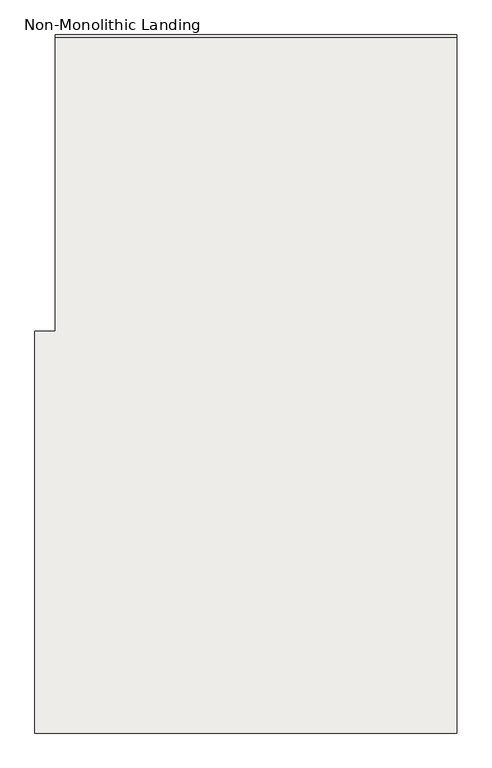
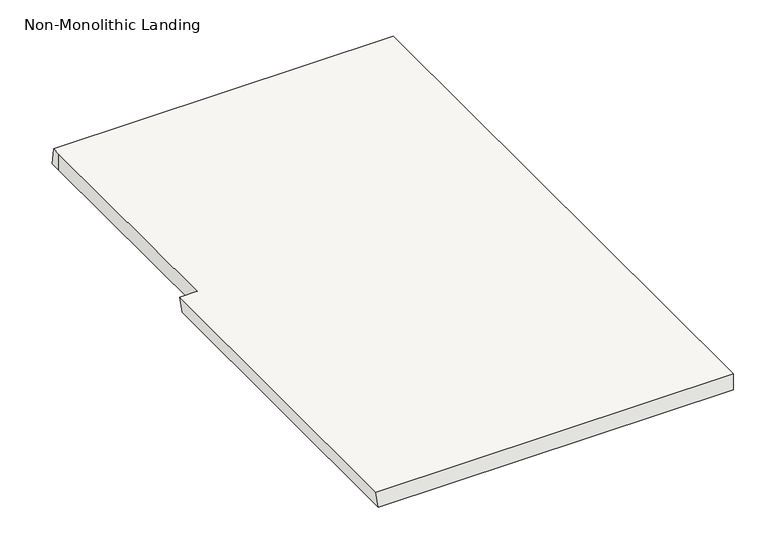
"""IFC4 building model written with IfcOpenShell, lengths in millimetres: slab geometry, Non-Monolithic Landing."""

from ifc_helpers import new_model, si_unit, origin, place, context, project, spatial, faceted_brep, source, transform, mapped, element, save


def non_monolithic_landing_00e8e037(model_context):
    return source(origin(), model_context, "Body", "Brep", [
        faceted_brep([(2075.213846, 2747.0262668, 1739.1304348), (3126.0396272, 2747.0262668, 1739.1304348), (3126.0396272, 4453.248464, 1739.1304348), (3126.0396272, 4478.248464, 1739.1304348), (2126.013846, 4478.248464, 1739.1304348), (2126.013846, 4453.248464, 1739.1304348), (2126.013846, 3747.052048, 1739.1304348), (2075.213846, 3747.052048, 1739.1304348), (3126.0396272, 4453.248464, 1689.1304348), (3126.0396272, 2747.0262668, 1689.1304348), (2082.401346, 2747.0262668, 1689.1304348), (2082.401346, 3747.052048, 1689.1304348), (2126.013846, 3747.052048, 1689.1304348), (2126.013846, 4453.248464, 1689.1304348), (2126.013846, 4485.435964, 1689.1304348), (3126.0396272, 4485.435964, 1689.1304348)], [[[0, 1, 2, 3, 4, 5, 6, 7]], [[8, 9, 10, 11, 12, 13, 14, 15]], [[1, 0, 10, 9]], [[3, 2, 8, 15]], [[5, 4, 14, 13]], [[6, 5, 13, 12]], [[3, 15, 14, 4]], [[2, 1, 9, 8]], [[7, 6, 12, 11]], [[0, 7, 11, 10]]]),
    ])


if __name__ == "__main__":
    model = new_model("IFC4")
    model_context = context("Model", 3, world=origin())
    ifc_project = project(units=[si_unit("LENGTHUNIT", "METRE", prefix="MILLI")], contexts=[model_context])
    site = spatial("IfcSite", under=ifc_project)
    building = spatial("IfcBuilding", under=site)
    placement = place(None, origin())
    non_monolithic_landing_shape = non_monolithic_landing_00e8e037(model_context)
    element("IfcSlab", 1, ObjectType="Non-Monolithic Landing", at=placement, inside=building, context=model_context, shape_type="MappedRepresentation", body=[
        mapped(non_monolithic_landing_shape, transform((0.0, 0.0, 0.0), x_axis=(1.0, 0.0, 0.0), y_axis=(0.0, 1.0, 0.0), z_axis=(0.0, 0.0, 1.0))),
    ])
    save(model, "model.ifc")
